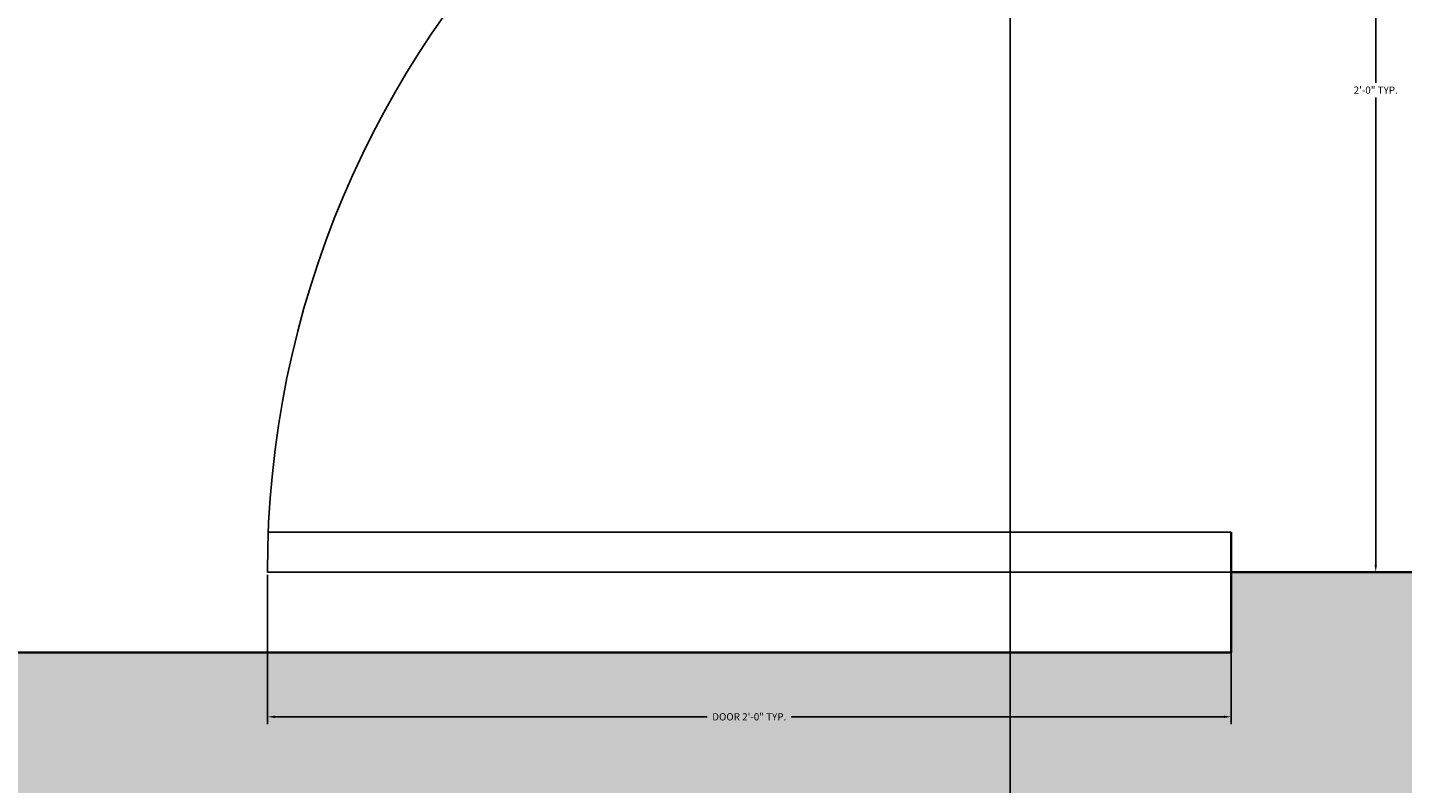
# Model space of a CAD drawing. Units: inches. Extents: x -5 to 482, y -460 to 66.
# Tile 19 of 31: x 120 to 154, y -143 to -124. Entities that reach past the tile are written whole.
import ezdxf

# ---------------------------------------------------------------- set-up
doc = ezdxf.new("R2010")
doc.units = ezdxf.units.IN
doc.header["$MEASUREMENT"] = 0
for name, color, linetype, lineweight in [('A-ANNO-DIMS', 2, 'Continuous', 18), ('A-DOOR', 3, 'Continuous', 25), ('A-WALL', 7, 'Continuous', 35), ('A-WALL-PATT', 152, 'Continuous', 13)]:
    doc.layers.add(name, color=color, linetype=linetype, lineweight=lineweight)
doc.styles.get("Standard").update_dxf_attribs({"font": 'arial.ttf'})
doc.dimstyles.get("Standard").update_dxf_attribs({"dimtxt": 0.18, "dimasz": 0.18, "dimexe": 0.18, "dimexo": 0.0625, "dimgap": 0.09, "dimtad": 0, "dimtih": 1, "dimtoh": 1, "dimdec": 0, "dimzin": 0, "dimdsep": 46, "dimlunit": 3, "dimtxsty": 'Standard', "dimcen": 0.09, "dimadec": 0, "dimazin": 0, "dimtfac": 1, "dimtdec": 0, "dimtofl": 0, "dimtmove": 0, "dimatfit": 3, "dimfxl": 1, "dimtolj": 1, "dimtzin": 0, "dimarcsym": 0})

# ---------------------------------------------------------------- blocks, each defined once
blk = doc.blocks.new('DOOR-SWING-24IN')
for p, q in [((24, 1), (0, 1)), ((24, 0), (0, 0))]:
    blk.add_line(p, q)
blk.add_arc((24, 0), 24, 90, 180)
blk = doc.blocks.new('*D41')
at = {"layer": 'A-ANNO-DIMS', "color": 0, "lineweight": -2, "transparency": 16777216}
for p, q in [((125.877, -137.911), (125.877, -141.629)), ((149.877, -137.911), (149.877, -141.629)), ((126.057, -141.449), (136.831, -141.449)), ((149.697, -141.449), (138.923, -141.449))]:
    blk.add_line(p, q, dxfattribs=at)
at = {"layer": 'A-ANNO-DIMS', "color": 0, "transparency": 16777216}
for points in [[(126.057, -141.419), (126.057, -141.479), (125.877, -141.449)], [(149.697, -141.419), (149.697, -141.479), (149.877, -141.449)]]:
    blk.add_solid(points, dxfattribs=at)
at = {"layer": 'Defpoints', "color": 0, "transparency": 16777216}
for p in [(125.877, -137.849), (149.877, -137.849), (149.877, -141.449)]:
    blk.add_point(p, dxfattribs=at)
at = {"layer": 'A-ANNO-DIMS', "color": 0, "transparency": 16777216, "insert": (137.877, -141.449), "char_height": 0.18, "attachment_point": 5}
blk.add_mtext('\\A1;DOOR 2\'-0" TYP.', dxfattribs=at)
blk = doc.blocks.new('*D42')
at = {"layer": 'A-ANNO-DIMS', "color": 0, "lineweight": -2, "transparency": 16777216}
for p, q in [((149.939, -113.849), (153.657, -113.849)), ((153.477, -114.029), (153.477, -125.667)), ((153.477, -137.669), (153.477, -126.031)), ((149.939, -137.849), (153.657, -137.849))]:
    blk.add_line(p, q, dxfattribs=at)
at = {"layer": 'A-ANNO-DIMS', "color": 0, "transparency": 16777216}
for points in [[(153.447, -114.029), (153.507, -114.029), (153.477, -113.849)], [(153.447, -137.669), (153.507, -137.669), (153.477, -137.849)]]:
    blk.add_solid(points, dxfattribs=at)
at = {"layer": 'Defpoints', "color": 0, "transparency": 16777216}
for p in [(149.877, -113.849), (153.477, -113.849), (149.877, -137.849)]:
    blk.add_point(p, dxfattribs=at)
at = {"layer": 'A-ANNO-DIMS', "color": 0, "transparency": 16777216, "insert": (153.477, -125.849), "char_height": 0.18, "attachment_point": 5}
blk.add_mtext('\\A1;2\'-0" TYP.', dxfattribs=at)
blk = doc.blocks.new('*D73')
at = {"layer": 'A-ANNO-DIMS', "color": 0, "lineweight": -2, "transparency": 16777216}
for p, q in [((144.377, -295.799), (144.377, 50.931)), ((144.557, 50.751), (160.976, 50.751)), ((178.197, 50.751), (161.777, 50.751)), ((178.377, -295.799), (178.377, 50.931))]:
    blk.add_line(p, q, dxfattribs=at)
at = {"layer": 'A-ANNO-DIMS', "color": 0, "transparency": 16777216}
for points in [[(144.557, 50.781), (144.557, 50.721), (144.377, 50.751)], [(178.197, 50.781), (178.197, 50.721), (178.377, 50.751)]]:
    blk.add_solid(points, dxfattribs=at)
at = {"layer": 'Defpoints', "color": 0, "transparency": 16777216}
for p in [(178.377, 50.751), (144.377, -295.861), (178.377, -295.861)]:
    blk.add_point(p, dxfattribs=at)
at = {"layer": 'A-ANNO-DIMS', "color": 0, "transparency": 16777216, "insert": (161.377, 50.751), "char_height": 0.18, "attachment_point": 5}
blk.add_mtext('\\A1;2\'-10"', dxfattribs=at)

msp = doc.modelspace()

# ---------------------------------------------------------------- hatches: boundary and pattern name
at = {"layer": 'A-WALL-PATT'}
h = msp.add_hatch(color=256, dxfattribs=at)
h.dxf.hatch_style = 1
h.paths.add_polyline_path([(149.377, -412.849), (144.377, -412.849), (144.377, -283.849), (144.377, -279.349), (133.877, -279.349), (133.877, -283.849), (139.877, -283.849), (139.877, -412.849), (133.51, -412.849), (133.51, -413.916), (102.652, -413.916), (102.652, -421.02), (133.51, -421.02), (133.51, -421.849), (149.377, -421.849)])
h.paths.add_polyline_path([(226.054, -412.849), (218.877, -412.849), (218.877, -350.849), (262.877, -350.849), (262.877, -386.849), (267.377, -386.849), (267.377, -283.849), (270.377, -283.849), (270.377, -279.349), (244.877, -279.349), (244.877, -283.849), (262.877, -283.849), (262.877, -346.349), (218.877, -346.349), (218.877, -283.849), (220.877, -283.849), (220.877, -279.349), (214.377, -279.349), (214.377, -283.849), (214.377, -412.849), (209.377, -412.849), (209.377, -421.849), (226.054, -421.849)])
h.paths.add_polyline_path([(315.815, -412.849), (250.054, -412.849), (250.054, -421.849), (315.815, -421.849)])
h.paths.add_polyline_path([(430.377, -378.349), (421.377, -378.349), (421.377, -412.849), (375.815, -412.849), (375.815, -421.849), (430.377, -421.849)])
h.paths.add_polyline_path([(78.691, -413.916), (47.68, -413.916), (47.68, -412.849), (41.877, -412.849), (41.877, -283.849), (109.877, -283.849), (109.877, -279.349), (41.877, -279.349), (41.877, -241.849), (32.877, -241.849), (32.877, -421.849), (47.68, -421.849), (47.68, -421.02), (78.691, -421.02)])
h.paths.add_polyline_path([(41.877, -144.349), (154.377, -144.349), (154.377, -137.849), (149.877, -137.849), (149.877, -139.849), (41.877, -139.849), (41.877, -97.849), (32.877, -97.849), (32.877, -181.849), (41.877, -181.849)])
h.paths.add_polyline_path([(430.377, -241.849), (421.377, -241.849), (421.377, -279.349), (309.377, -279.349), (309.377, -170.349), (304.877, -170.349), (304.877, -279.349), (294.377, -279.349), (294.377, -283.849), (421.377, -283.849), (421.377, -318.349), (430.377, -318.349)])
h.paths.add_polyline_path([(430.377, -119.849), (421.377, -119.849), (421.377, -139.849), (419.377, -139.849), (419.377, -144.349), (421.377, -144.349), (421.377, -181.849), (430.377, -181.849)])
h.paths.add_polyline_path([(395.377, -139.849), (377.377, -139.849), (377.377, -75.849), (421.377, -75.849), (421.377, -95.849), (430.377, -95.849), (430.377, -45.599), (421.377, -45.599), (421.377, -71.349), (377.377, -71.349), (377.377, -22.849), (372.877, -22.849), (372.877, -139.849), (242.877, -139.849), (242.877, -137.849), (238.377, -137.849), (238.377, -144.349), (304.877, -144.349), (304.877, -146.349), (309.377, -146.349), (309.377, -144.349), (395.377, -144.349)])
h.paths.add_polyline_path([(65.877, 13.151), (32.877, 13.151), (32.877, -37.849), (41.877, -37.849), (41.877, 4.151), (65.877, 4.151)])
h.paths.add_polyline_path([(166.377, 13.151), (125.877, 13.151), (125.877, 4.151), (149.877, 4.151), (149.877, -113.849), (154.377, -113.849), (154.377, 4.151), (166.377, 4.151)])
h.paths.add_polyline_path([(277.877, 13.151), (226.377, 13.151), (226.377, 4.151), (238.377, 4.151), (238.377, -113.849), (242.877, -113.849), (242.877, 4.151), (277.877, 4.151)])
h.paths.add_polyline_path([(430.377, 13.151), (337.877, 13.151), (337.877, 4.151), (372.877, 4.151), (372.877, 1.151), (377.377, 1.151), (377.377, 4.151), (421.377, 4.151), (421.377, -21.599), (430.377, -21.599)])

# ---------------------------------------------------------------- linework, layer by layer
at = {"layer": 'A-WALL'}
for p, q in [((149.877, -136.849), (149.877, -139.849)), ((149.877, -137.849), (154.377, -137.849)), ((41.877, -139.849), (149.877, -139.849))]:
    msp.add_line(p, q, dxfattribs=at)

# ---------------------------------------------------------------- block references
at = {"layer": 'A-DOOR'}
msp.add_blockref('DOOR-SWING-24IN', (125.877, -137.849), dxfattribs=at)

# ---------------------------------------------------------------- dimensions: what is measured, and where the dimension line sits
at = {"layer": 'A-ANNO-DIMS'}
dim = msp.add_linear_dim(base=(178.377, 50.751), p1=(144.377, -295.861), p2=(178.377, -295.861), dimstyle='Standard', override={"dimdec": 1, "dimlfac": 1, "dimrnd": 0, "dimzin": 1, "dimdsep": 46, "dimlunit": 4, "dimfrac": 2}, dxfattribs=at)
dim.commit()
dim.dimension.update_dxf_attribs({"geometry": '*D73', "text_midpoint": (161.377, 50.751)})
dim = msp.add_linear_dim(base=(153.477, -113.849), p1=(149.877, -137.849), p2=(149.877, -113.849), angle=90, text='<> TYP.', dimstyle='Standard', override={"dimdec": 1, "dimlfac": 1, "dimrnd": 0, "dimzin": 1, "dimdsep": 46, "dimlunit": 4, "dimfrac": 2}, dxfattribs=at)
dim.commit()
dim.dimension.update_dxf_attribs({"geometry": '*D42', "text_midpoint": (153.477, -125.849)})
dim = msp.add_linear_dim(base=(149.877, -141.449), p1=(125.877, -137.849), p2=(149.877, -137.849), text='DOOR <> TYP.', dimstyle='Standard', override={"dimdec": 1, "dimlfac": 1, "dimrnd": 0, "dimzin": 1, "dimdsep": 46, "dimlunit": 4, "dimfrac": 2}, dxfattribs=at)
dim.commit()
dim.dimension.update_dxf_attribs({"geometry": '*D41', "text_midpoint": (137.877, -141.449)})

doc.saveas('drawing.dxf')
